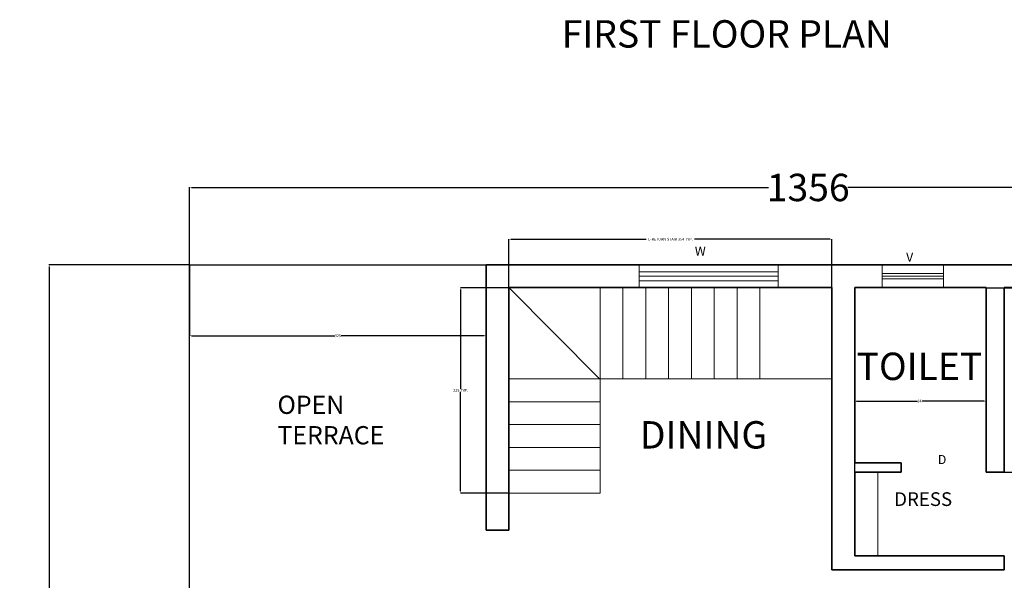
# Model space of a CAD drawing. Units: centimetres. Extents: x -121 to 3851, y -16 to 1180.
# Tile 13 of 16: x 2225 to 3304, y 566 to 1180. Entities that reach past the tile are written whole.
import ezdxf

# ---------------------------------------------------------------- set-up
doc = ezdxf.new("R2010")
doc.units = ezdxf.units.CM
doc.header["$MEASUREMENT"] = 0
for name, color, linetype, lineweight in [('A-ANNO-DIMS', 2, 'Continuous', 18), ('A-ANNO-IDEN', 3, 'Continuous', 13), ('A-ANNO-TEXT', 7, 'Continuous', 25), ('A-AREA-IDEN', 3, 'Continuous', 18), ('A-FLOR', 8, 'Continuous', 25), ('A-FLOR-CASE', 9, 'Continuous', 18), ('A-FLOR-STRS', 3, 'Continuous', 18), ('A-GLAZ', 4, 'Continuous', 18), ('A-WALL', 7, 'Continuous', 35)]:
    doc.layers.add(name, color=color, linetype=linetype, lineweight=lineweight)
doc.styles.get("Standard").update_dxf_attribs({"font": 'arial.ttf'})
doc.dimstyles.get("Standard").update_dxf_attribs({"dimtxt": 3, "dimasz": 2, "dimexe": 0.18, "dimexo": 0.0625, "dimgap": 0.09, "dimtad": 0, "dimtih": 1, "dimtoh": 1, "dimdec": 0, "dimzin": 0, "dimdsep": 46, "dimtxsty": 'Standard', "dimcen": 0.09, "dimadec": 0, "dimazin": 0, "dimtfac": 1, "dimtdec": 0, "dimtofl": 0, "dimtmove": 0, "dimatfit": 3, "dimfxl": 1, "dimtolj": 1, "dimtzin": 0, "dimarcsym": 0})

# ---------------------------------------------------------------- blocks, each defined once
blk = doc.blocks.new('*D16')
at = {"layer": 'A-ANNO-DIMS', "color": 0, "lineweight": -2, "transparency": 16777216}
for p, q in [((2411.3, 911.8), (2411.3, 996.7)), ((2413.3, 996.5), (3045.8, 996.5)), ((3765.3, 996.5), (3132.7, 996.5)), ((3767.3, 911.8), (3767.3, 996.7))]:
    blk.add_line(p, q, dxfattribs=at)
at = {"layer": 'A-ANNO-DIMS', "color": 0, "transparency": 16777216}
for points in [[(2413.3, 996.8), (2413.3, 996.1), (2411.3, 996.5)], [(3765.3, 996.8), (3765.3, 996.1), (3767.3, 996.5)]]:
    blk.add_solid(points, dxfattribs=at)
at = {"layer": 'Defpoints', "color": 0, "transparency": 16777216}
for p in [(3767.3, 996.5), (2411.3, 911.7), (3767.3, 911.7)]:
    blk.add_point(p, dxfattribs=at)
at = {"layer": 'A-ANNO-DIMS', "color": 0, "transparency": 16777216, "insert": (3089.3, 996.5), "char_height": 3, "attachment_point": 5}
blk.add_mtext('\\A1;{\\H10x;1356}', dxfattribs=at)
blk = doc.blocks.new('*D13')
at = {"layer": 'A-ANNO-DIMS', "color": 0, "lineweight": -2, "transparency": 16777216}
for p, q in [((2411.2, 911.7), (2257, 911.7)), ((2257.2, 909.7), (2257.2, 519.1)), ((2257.2, 97.7), (2257.2, 488.3)), ((2411.2, 95.7), (2257, 95.7))]:
    blk.add_line(p, q, dxfattribs=at)
at = {"layer": 'A-ANNO-DIMS', "color": 0, "transparency": 16777216}
for points in [[(2256.9, 909.7), (2257.5, 909.7), (2257.2, 911.7)], [(2256.9, 97.7), (2257.5, 97.7), (2257.2, 95.7)]]:
    blk.add_solid(points, dxfattribs=at)
at = {"layer": 'Defpoints', "color": 0, "transparency": 16777216}
for p in [(2411.3, 911.7), (2257.2, 95.7), (2411.3, 95.7)]:
    blk.add_point(p, dxfattribs=at)
at = {"layer": 'A-ANNO-DIMS', "color": 0, "transparency": 16777216, "insert": (2257.2, 503.7), "char_height": 3, "attachment_point": 5}
blk.add_mtext('\\A1;{\\H10x;816}', dxfattribs=at)
blk = doc.blocks.new('WIN-152CM')
for p, q in [((0, 17.5), (152.2, 17.5)), ((0, 12.5), (152.2, 12.5)), ((0, 7.5), (152.2, 7.5))]:
    blk.add_line(p, q)
blk.add_lwpolyline([(0, 25), (152.2, 25), (152.2, 0), (0, 0)], close=True)
blk = doc.blocks.new('VENT-67CM')
for p, q in [((0, 15.5), (67.3, 15.5)), ((0, 12.5), (67.3, 12.5)), ((0, 9.5), (67.3, 9.5))]:
    blk.add_line(p, q)
blk.add_lwpolyline([(0, 25), (67.3, 25), (67.3, 0), (0, 0)], close=True)
blk = doc.blocks.new('STAIR-L-RETURN')
for p, q in [((0, 225), (99.1, 125)), ((100, 100), (100, 225)), ((125, 125), (125, 225)), ((150, 125), (150, 225)), ((175, 125), (175, 225)), ((200, 125), (200, 225)), ((225, 125), (225, 225)), ((250, 125), (250, 225)), ((275, 125), (275, 225)), ((0, 125), (99.1, 125)), ((99.1, 125), (354, 125)), ((100, 0), (100, 125)), ((0, 100), (100, 100)), ((0, 75), (100, 75)), ((0, 50), (100, 50)), ((0, 25), (100, 25)), ((0, 0), (100, 0))]:
    blk.add_line(p, q)
blk = doc.blocks.new('*D33')
at = {"layer": 'A-ANNO-DIMS', "color": 0, "lineweight": -2, "transparency": 16777216}
for p, q in [((2761.3, 886.8), (2761.3, 940)), ((2763.3, 939.8), (2911.8, 939.8)), ((3113.3, 939.8), (2964.7, 939.8)), ((3115.3, 886.8), (3115.3, 940))]:
    blk.add_line(p, q, dxfattribs=at)
at = {"layer": 'A-ANNO-DIMS', "color": 0, "transparency": 16777216}
for points in [[(2763.3, 940.2), (2763.3, 939.5), (2761.3, 939.8)], [(3113.3, 940.2), (3113.3, 939.5), (3115.3, 939.8)]]:
    blk.add_solid(points, dxfattribs=at)
at = {"layer": 'Defpoints', "color": 0, "transparency": 16777216}
for p in [(3115.3, 939.8), (2761.3, 886.7), (3115.3, 886.7)]:
    blk.add_point(p, dxfattribs=at)
at = {"layer": 'A-ANNO-DIMS', "color": 0, "transparency": 16777216, "insert": (2938.3, 939.8), "char_height": 3, "attachment_point": 5}
blk.add_mtext('\\A1;L-RETURN STAIR 354 TYP.', dxfattribs=at)
blk = doc.blocks.new('*D34')
at = {"layer": 'A-ANNO-DIMS', "color": 0, "lineweight": -2, "transparency": 16777216}
for p, q in [((2761.2, 886.7), (2708, 886.7)), ((2708.2, 884.7), (2708.2, 775.8)), ((2708.2, 663.7), (2708.2, 772.6)), ((2761.2, 661.7), (2708, 661.7))]:
    blk.add_line(p, q, dxfattribs=at)
at = {"layer": 'A-ANNO-DIMS', "color": 0, "transparency": 16777216}
for points in [[(2707.8, 884.7), (2708.5, 884.7), (2708.2, 886.7)], [(2707.8, 663.7), (2708.5, 663.7), (2708.2, 661.7)]]:
    blk.add_solid(points, dxfattribs=at)
at = {"layer": 'Defpoints', "color": 0, "transparency": 16777216}
for p in [(2708.2, 886.7), (2761.3, 886.7), (2761.3, 661.7)]:
    blk.add_point(p, dxfattribs=at)
at = {"layer": 'A-ANNO-DIMS', "color": 0, "transparency": 16777216, "insert": (2708.2, 774.2), "char_height": 3, "attachment_point": 5}
blk.add_mtext('\\A1;225 TYP.', dxfattribs=at)
blk = doc.blocks.new('*D65')
at = {"layer": 'A-ANNO-DIMS', "color": 0, "lineweight": -2, "transparency": 16777216}
for p, q in [((2411.3, 911.7), (2411.3, 833.8)), ((2736.3, 911.7), (2736.3, 833.8)), ((2413.3, 834), (2570.3, 834)), ((2734.3, 834), (2577.2, 834))]:
    blk.add_line(p, q, dxfattribs=at)
at = {"layer": 'A-ANNO-DIMS', "color": 0, "transparency": 16777216}
for points in [[(2413.3, 834.3), (2413.3, 833.6), (2411.3, 834)], [(2734.3, 834.3), (2734.3, 833.6), (2736.3, 834)]]:
    blk.add_solid(points, dxfattribs=at)
at = {"layer": 'Defpoints', "color": 0, "transparency": 16777216}
for p in [(2411.3, 911.7), (2736.3, 911.7), (2411.3, 834)]:
    blk.add_point(p, dxfattribs=at)
at = {"layer": 'A-ANNO-DIMS', "color": 0, "transparency": 16777216, "insert": (2573.8, 834), "char_height": 3, "attachment_point": 5}
blk.add_mtext('\\A1;325', dxfattribs=at)
blk = doc.blocks.new('*D68')
at = {"layer": 'A-ANNO-DIMS', "color": 0, "lineweight": -2, "transparency": 16777216}
for p, q in [((3140.3, 684.8), (3140.3, 762.7)), ((3142.3, 762.5), (3209, 762.5)), ((3282.3, 762.5), (3215.5, 762.5)), ((3284.3, 684.8), (3284.3, 762.7))]:
    blk.add_line(p, q, dxfattribs=at)
at = {"layer": 'A-ANNO-DIMS', "color": 0, "transparency": 16777216}
for points in [[(3142.3, 762.8), (3142.3, 762.1), (3140.3, 762.5)], [(3282.3, 762.8), (3282.3, 762.1), (3284.3, 762.5)]]:
    blk.add_solid(points, dxfattribs=at)
at = {"layer": 'Defpoints', "color": 0, "transparency": 16777216}
for p in [(3284.3, 762.5), (3140.3, 684.7), (3284.3, 684.7)]:
    blk.add_point(p, dxfattribs=at)
at = {"layer": 'A-ANNO-DIMS', "color": 0, "transparency": 16777216, "insert": (3212.3, 762.5), "char_height": 3, "attachment_point": 5}
blk.add_mtext('\\A1;144', dxfattribs=at)
blk = doc.blocks.new('*D69')
at = {"layer": 'A-ANNO-DIMS', "color": 0, "lineweight": -2, "transparency": 16777216}
for p, q in [((3284.3, 886.7), (3362.2, 886.7)), ((3362, 884.7), (3362, 787.3)), ((3362, 686.7), (3362, 784.1)), ((3284.3, 684.7), (3362.2, 684.7))]:
    blk.add_line(p, q, dxfattribs=at)
at = {"layer": 'A-ANNO-DIMS', "color": 0, "transparency": 16777216}
for points in [[(3361.7, 884.7), (3362.3, 884.7), (3362, 886.7)], [(3361.7, 686.7), (3362.3, 686.7), (3362, 684.7)]]:
    blk.add_solid(points, dxfattribs=at)
at = {"layer": 'Defpoints', "color": 0, "transparency": 16777216}
for p in [(3284.3, 886.7), (3284.3, 684.7), (3362, 684.7)]:
    blk.add_point(p, dxfattribs=at)
at = {"layer": 'A-ANNO-DIMS', "color": 0, "transparency": 16777216, "insert": (3362, 785.7), "char_height": 3, "attachment_point": 5}
blk.add_mtext('\\A1;202', dxfattribs=at)

msp = doc.modelspace()

# ---------------------------------------------------------------- linework, layer by layer
at = {"layer": 'A-FLOR'}
for p, q in [((2411.2642, 911.7228), (2736.2642, 911.7228)), ((2411.2642, 95.7228), (2411.2642, 911.7228))]:
    msp.add_line(p, q, dxfattribs=at)
at = {"layer": 'A-FLOR-CASE'}
msp.add_line((3165.7533, 684.7228), (3165.7533, 592.7228), dxfattribs=at)
at = {"layer": 'A-WALL'}
for p, q in [((2736.2642, 911.7228), (3767.2642, 911.7228)), ((2736.2642, 886.7228), (2736.2642, 911.7228)), ((2736.2642, 709.7228), (2736.2642, 886.7228)), ((2761.2642, 886.7228), (3115.2642, 886.7228)), ((2761.2642, 620.9935), (2761.2642, 886.7228)), ((3115.2642, 886.7228), (3115.2642, 577.7228)), ((3140.2642, 886.7228), (3284.2642, 886.7228)), ((3140.2642, 886.7228), (3140.2642, 694.7228)), ((3284.2642, 886.7228), (3284.2642, 684.7228)), ((3304.2642, 886.7228), (3742.2642, 886.7228)), ((3304.2642, 886.7228), (3304.2642, 684.7228)), ((2736.2642, 620.9935), (2736.2642, 709.7228)), ((3140.2642, 694.7228), (3191.2424, 694.7228)), ((3191.2424, 694.7228), (3191.2424, 684.7228)), ((3140.2642, 684.7228), (3191.2424, 684.7228)), ((3140.2642, 684.7228), (3140.2642, 592.7228)), ((3284.2642, 684.7228), (3304.2642, 684.7228)), ((2736.2642, 620.9935), (2761.2642, 620.9935)), ((3140.2642, 592.7228), (3304.2642, 592.7228)), ((3304.2642, 592.7228), (3304.2642, 577.7228)), ((3115.2642, 577.7228), (3304.2642, 577.7228))]:
    msp.add_line(p, q, dxfattribs=at)

# ---------------------------------------------------------------- block references
at = {"layer": 'A-FLOR-STRS'}
msp.add_blockref('STAIR-L-RETURN', (2761.264, 661.7227), dxfattribs=at)
at = {"layer": 'A-GLAZ'}
for name, p in [('WIN-152CM', (2904.0565, 886.7227)), ('VENT-67CM', (3170.199, 886.7227))]:
    msp.add_blockref(name, p, dxfattribs=at)

# ---------------------------------------------------------------- texts
at = {"layer": 'A-ANNO-IDEN', "char_height": 10, "attachment_point": 1}
for s, insert in [('W', (2965.0273, 931.7614)), ('V', (3196.6006, 925.22)), ('D', (3231.3605, 703.3876))]:
    msp.add_mtext_dynamic_manual_height_columns(s, width=55.718495, gutter_width=1, heights=[0], dxfattribs=dict(at, insert=insert))
at = {"layer": 'A-ANNO-TEXT', "insert": (2819.0916, 1179.8042), "char_height": 30, "attachment_point": 1}
msp.add_mtext_dynamic_manual_height_columns('FIRST FLOOR PLAN', width=1207.704783, gutter_width=1, heights=[0], dxfattribs=at)
at = {"layer": 'A-AREA-IDEN', "attachment_point": 1}
for s, width, insert, char_height in [('TOILET', 114.065148, (3142.3758, 815.5188), 30), ('OPEN TERRACE', 143.846156, (2507.5049, 768.3761), 20), ('DINING', 149.976594, (2904.7938, 740.4511), 30), ('DRESS', 14.894434, (3183.536, 662.5167), 15)]:
    msp.add_mtext_dynamic_manual_height_columns(s, width=width, gutter_width=1, heights=[0], dxfattribs=dict(at, insert=insert, char_height=char_height))

# ---------------------------------------------------------------- dimensions: what is measured, and where the dimension line sits
at = {"layer": 'A-ANNO-DIMS'}
for base, p1, p2, text, override, picture, middle in [((3767.2642, 996.4769), (2411.2642, 911.7228), (3767.2642, 911.7228), '{\\H10x;<>}', {"dimclrd": 0, "dimclre": 0, "dimclrt": 0}, '*D16', (3089.2642, 996.4769)), ((3115.2642, 939.8228), (2761.2642, 886.7228), (3115.2642, 886.7228), 'L-RETURN STAIR <> TYP.', {"dimdec": 0, "dimlfac": 1, "dimrnd": 0, "dimzin": 0, "dimdsep": 46, "dimlunit": 2}, '*D33', (2938.2642, 939.8228))]:
    dim = msp.add_linear_dim(base=base, p1=p1, p2=p2, text=text, dimstyle='Standard', override=override, dxfattribs=at)
    dim.commit()
    dim.dimension.update_dxf_attribs({"geometry": picture, "text_midpoint": middle})
for base, p1, p2, text, override, picture, middle in [((2257.1851, 95.7228), (2411.2642, 911.7228), (2411.2642, 95.7228), '{\\H10x;<>}', {"dimclrd": 0, "dimclre": 0, "dimclrt": 0}, '*D13', (2257.1851, 503.7228)), ((2708.1642, 886.7228), (2761.2642, 661.7228), (2761.2642, 886.7228), '<> TYP.', {"dimdec": 0, "dimlfac": 1, "dimrnd": 0, "dimzin": 0, "dimdsep": 46, "dimlunit": 2}, '*D34', (2708.1642, 774.2228))]:
    dim = msp.add_linear_dim(base=base, p1=p1, p2=p2, angle=90, text=text, dimstyle='Standard', override=override, dxfattribs=at)
    dim.commit()
    dim.dimension.update_dxf_attribs({"geometry": picture, "text_midpoint": middle})
for base, p1, p2, angle, picture, middle in [((2411.2642, 833.9728), (2736.2642, 911.7228), (2411.2642, 911.7228), 180, '*D65', (2573.7642, 833.9728)), ((3362.0142, 684.7228), (3284.2642, 886.7228), (3284.2642, 684.7228), 270, '*D69', (3362.0142, 785.7228))]:
    dim = msp.add_linear_dim(base=base, p1=p1, p2=p2, angle=angle, dimstyle='Standard', override={"dimdec": 0, "dimlfac": 1, "dimrnd": 0, "dimzin": 0, "dimdsep": 46, "dimlunit": 2}, dxfattribs=at)
    dim.commit()
    dim.dimension.update_dxf_attribs({"geometry": picture, "text_midpoint": middle})
dim = msp.add_linear_dim(base=(3284.2642, 762.4728), p1=(3140.2642, 684.7228), p2=(3284.2642, 684.7228), dimstyle='Standard', override={"dimdec": 0, "dimlfac": 1, "dimrnd": 0, "dimzin": 0, "dimdsep": 46, "dimlunit": 2}, dxfattribs=at)
dim.commit()
dim.dimension.update_dxf_attribs({"geometry": '*D68', "text_midpoint": (3212.2642, 762.4728)})

doc.saveas('drawing.dxf')
